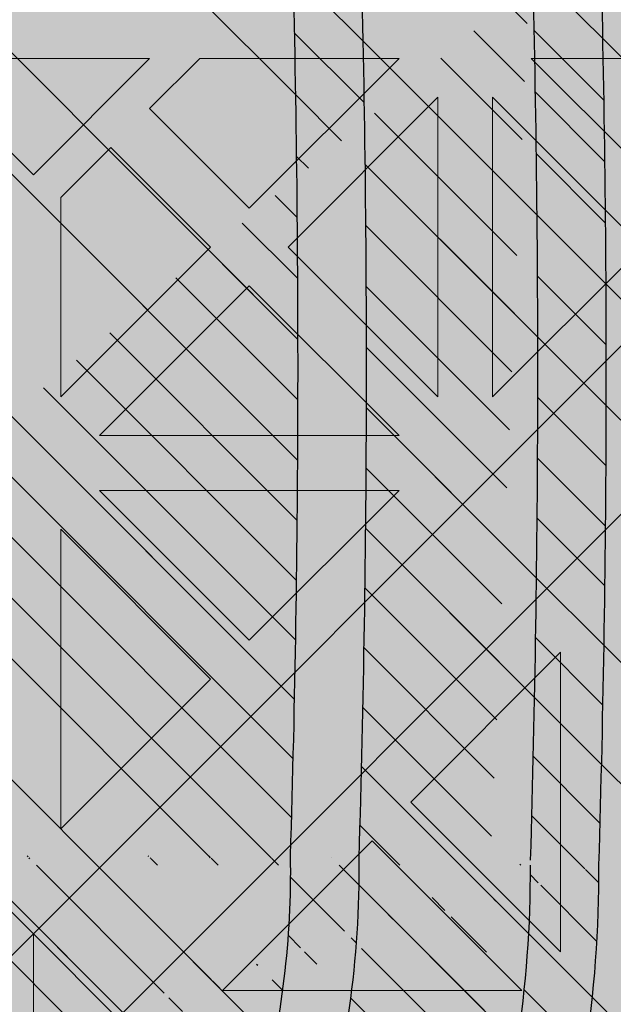
# Model space of a CAD drawing. Units: inches. Extents: x 844 to 2234, y 346 to 1084.
# Tile 28 of 93: x 1257.311 to 1260.074, y 691.183 to 695.763. Entities that reach past the tile are written whole.
import ezdxf

# ---------------------------------------------------------------- set-up
doc = ezdxf.new("R2010")
doc.units = ezdxf.units.IN
doc.header["$MEASUREMENT"] = 0
doc.layers.add('furniture', color=8, linetype='Continuous', lineweight=18)
doc.layers.add('RA-AP-01$0$INT', color=35, linetype='Continuous', lineweight=5)
doc.layers.add('RA-AP-01$0$FURN', color=3, linetype='Continuous')
doc.layers.add('RA-AP-01$0$WOOD', color=64, linetype='Continuous')

# ---------------------------------------------------------------- blocks, each defined once
blk = doc.blocks.new('A$C18D01794')
at = {"layer": 'RA-AP-01$0$INT'}
h = blk.add_hatch(color=256, dxfattribs=at)
h.paths.add_polyline_path([(4.585917135068449, -6.356712009588271), (4.555206456959269, -6.35671200958746), (4.555206456959137, -6.387422687716308), (4.874495778835233, -6.706712009592356), (4.90520645695423, -6.676001331474049)])
h.paths.add_polyline_path([(5.255206456948813, -6.387422687716306), (5.255206456948682, -6.356712009605972), (5.224495778822613, -6.356712009605161), (4.905206456953498, -6.676001331474273), (4.935917135072151, -6.706712009592924)])
h.paths.add_polyline_path([(4.935917135072559, -6.706712009592068), (4.905206456953564, -6.737422687710376), (5.255206456951813, -7.087422687708613), (5.255206456951549, -7.026001331471008)])
h.paths.add_polyline_path([(4.555206456956399, -7.026001331471013), (4.555206456956134, -7.087422687708616), (4.905206456953821, -6.737422687710943), (4.874495778835166, -6.70671200959229)])
h = blk.add_hatch(color=256, dxfattribs=at)
h.paths.add_polyline_path([(4.585917135068448, -6.356712009588273), (4.614201406330596, -6.356712009589021), (4.668846067270487, -6.411356670531338), (4.723490728212344, -6.356712009591912), (4.771774999457151, -6.35671200959319), (4.826419660396886, -6.411356670535356), (4.862780050090322, -6.374996280843536), (4.844495778842715, -6.356712009595112), (4.862780050090411, -6.356712009595595), (4.905206456960182, -6.399138416468211), (4.947632863832445, -6.356712009597838), (4.965917135079675, -6.356712009598322), (4.947632863831759, -6.374996280845421), (4.983993253523576, -6.411356670538857), (5.038637914464627, -6.356712009600247), (5.08692218571208, -6.356712009601523), (5.141566846649976, -6.411356670541852), (5.196211507589851, -6.356712009604411), (5.224495778822615, -6.356712009605161), (4.905206456953975, -6.676001331473793)])
h.paths.add_polyline_path([(4.895206456956031, -6.637717060225675), (4.895206456958921, -6.528427738347902), (4.840561796018589, -6.583072399285802)], flags=16)
h.paths.add_polyline_path([(4.915206456955638, -6.637717060226121), (4.969851117895509, -6.583072399288678), (4.915206456957609, -6.528427738348344)], flags=16)
h.paths.add_polyline_path([(4.826419660395175, -6.568930263661755), (4.881064321335613, -6.514285602723745), (4.771774999456703, -6.514285602720857)], flags=16)
h.paths.add_polyline_path([(4.983993253519558, -6.568930263665262), (5.038637914460456, -6.514285602726792), (4.929348592581548, -6.514285602724816)], flags=16)
h.paths.add_polyline_path([(4.881064321336025, -6.494285602723742), (4.826419660397532, -6.439640941782821), (4.771774999457062, -6.494285602720859)], flags=16)
h.paths.add_polyline_path([(4.929348592582019, -6.494285602724817), (5.038637914460982, -6.494285602726792), (4.983993253522945, -6.439640941786327)], flags=16)
h.paths.add_polyline_path([(4.895206456960191, -6.480143467100443), (4.895206456962115, -6.407422687715913), (4.876922185715016, -6.389138416467584), (4.840561796021581, -6.425498806159401)], flags=16)
h.paths.add_polyline_path([(4.915206456958487, -6.480143467100889), (4.969851117899527, -6.425498806162279), (4.933490728206909, -6.389138416468043), (4.9152064569598, -6.40742268771434)], flags=16)
h.paths.add_polyline_path([(4.757632863832376, -6.480143467096812), (4.812277524772842, -6.425498806158772), (4.757632863834348, -6.370854145217844)], flags=16)
h.paths.add_polyline_path([(4.737632863832376, -6.480143467096286), (4.737632863834348, -6.370854145217375), (4.682988202893906, -6.425498806155385)], flags=16)
h.paths.add_polyline_path([(5.05278005008503, -6.480143467103376), (5.052780050087917, -6.370854145224413), (4.998135389146995, -6.425498806162908)], flags=16)
h.paths.add_polyline_path([(5.072780050085024, -6.480143467103744), (5.127424711025931, -6.42549880616527), (5.072780050087916, -6.370854145224832)], flags=16)
h.paths.add_polyline_path([(4.935917135072783, -6.706712009592292), (5.255206456948811, -6.387422687716309), (5.255206456948932, -6.415706958964177), (5.200561796010279, -6.470351619902839), (5.255206456949403, -6.524996280841948), (5.25520645694961, -6.5732805520894), (5.200561796009787, -6.627925213029239), (5.236922185702417, -6.664285602721864), (5.255206456949919, -6.646001331474357), (5.255206456949998, -6.664285602721898), (5.212780050078687, -6.706712009592262), (5.25520645695036, -6.749138416463932), (5.255206456950438, -6.767422687711313), (5.236922185702424, -6.749138416463297), (5.200561796009796, -6.785498806155928), (5.255206456950753, -6.840143467096874), (5.25520645695096, -6.888427738341682), (5.200561796010322, -6.943072399282328), (5.255206456951428, -6.997717060223427), (5.255206456951547, -7.026001331471006)])
h.paths.add_polyline_path([(5.042988202883395, -6.785498806155427), (5.097632863823085, -6.840143467095101), (5.097632863822622, -6.730854145216193)], flags=16)
h.paths.add_polyline_path([(5.028846067259663, -6.771356670531693), (5.083490728198774, -6.716712009592573), (4.974201406321001, -6.716712009593042)], flags=16)
h.paths.add_polyline_path([(5.117632863823087, -6.840143467095186), (5.172277524762331, -6.785498806155926), (5.11763286382262, -6.730854145216225)], flags=16)
h.paths.add_polyline_path([(5.08349072819877, -6.696712009593886), (5.028846067259652, -6.642067348654775), (4.974201406320998, -6.696712009593438)], flags=16)
h.paths.add_polyline_path([(5.131774999446817, -6.854285602718917), (5.186419660386065, -6.799640941779662), (5.241064321325782, -6.854285602719365)], flags=17)
h.paths.add_polyline_path([(5.131774999446228, -6.716712009592374), (5.186419660386065, -6.771356670532194), (5.222780050079488, -6.734996280838764), (5.204495778832781, -6.716712009592063)], flags=16)
h.paths.add_polyline_path([(5.097632863822613, -6.682569873970264), (5.097632863823061, -6.573280552091354), (5.042988202883383, -6.627925213031044)], flags=16)
h.paths.add_polyline_path([(5.131774999446899, -6.874285602718915), (5.241064321325809, -6.874285602719364), (5.186419660386591, -6.928930263658598)], flags=17)
h.paths.add_polyline_path([(5.131774999446226, -6.696712009594078), (5.204495778830767, -6.696712009594374), (5.22278005007868, -6.67842773834687), (5.186419660386049, -6.642067348654249)], flags=16)
h.paths.add_polyline_path([(5.11763286382262, -6.682569873970225), (5.17227752476232, -6.627925213030515), (5.117632863823064, -6.573280552091267)], flags=16)
h.paths.add_polyline_path([(5.186419660386069, -6.613783077405491), (5.241064321325754, -6.559138416465795), (5.131774999446791, -6.559138416466263)], flags=16)
h.paths.add_polyline_path([(5.131774999446872, -6.539138416466263), (5.24106432132578, -6.539138416465794), (5.186419660386554, -6.484493755526573)], flags=16)
h.paths.add_polyline_path([(5.255206456951811, -7.08742268770861), (5.255206456951895, -7.106712009588038), (4.555206456956052, -7.106712009588038), (4.555206456956136, -7.087422687708617), (4.905206456953973, -6.737422687710788)])
h.paths.add_polyline_path([(4.983993253513404, -6.8444937555241), (4.92934859257295, -6.899138416462108), (5.03863791445186, -6.899138416465014)], flags=16)
h.paths.add_polyline_path([(4.969851117889988, -6.83035161990006), (4.915206456952556, -6.775706958960171), (4.915206456949648, -6.884996280837944)], flags=16)
h.paths.add_polyline_path([(4.929348592572535, -6.919138416462105), (4.983993253511019, -6.973783077403037), (5.038637914451496, -6.919138416465012)], flags=16)
h.paths.add_polyline_path([(5.052780050074912, -6.93328055208906), (4.998135389134438, -6.987925213027088), (5.052780050072919, -7.042569873968025)], flags=16)
h.paths.add_polyline_path([(5.07278005007491, -6.933280552089588), (5.072780050072918, -7.042569873968497), (5.127424711013374, -6.987925213030498)], flags=16)
h.paths.add_polyline_path([(4.89520645695295, -6.775706958959721), (4.840561796013067, -6.830351619897157), (4.895206456950961, -6.884996280837494)], flags=16)
h.paths.add_polyline_path([(4.915206456948365, -6.933280552085403), (4.915206456946434, -7.006001331471951), (4.933490728192729, -7.024285602719066), (4.969851117886972, -6.987925213026453)], flags=16)
h.paths.add_polyline_path([(4.881064321327021, -6.899138416461022), (4.82641966038902, -6.84449375552057), (4.771774999448108, -6.899138416459029)], flags=16)
h.paths.add_polyline_path([(4.895206456950073, -6.933280552084951), (4.840561796009022, -6.987925213023558), (4.876922185700835, -7.024285602716997), (4.895206456948749, -7.006001331469487)], flags=16)
h.paths.add_polyline_path([(4.983993253510392, -7.0020673486505), (4.947632863816944, -7.038427738342319), (4.965917135064043, -7.05671200959023), (5.038637914448995, -7.056712009591555)], flags=16)
h.paths.add_polyline_path([(4.881064321326543, -6.91913841646102), (4.771774999447578, -6.919138416459031), (4.826419660385607, -6.973783077399508)], flags=16)
h.paths.add_polyline_path([(4.905206456946447, -7.014285602717636), (4.862780050074785, -7.056712009588352), (4.947632863816685, -7.056712009589775)], flags=16)
h.paths.add_polyline_path([(5.14156684663679, -7.002067348654549), (5.086922185696452, -7.056712009592438), (5.196211507574223, -7.056712009594425)], flags=16)
h.paths.add_polyline_path([(4.8264196603837, -7.002067348646972), (4.771774999442643, -7.056712009585575), (4.8444957788276, -7.056712009587508), (4.862780050075511, -7.038427738340416)], flags=16)
h.paths.add_polyline_path([(4.812277524760289, -6.98792521302292), (4.757632863822258, -6.933280552082447), (4.757632863819352, -7.042569873961408)], flags=16)
h.paths.add_polyline_path([(4.73763286382226, -6.933280552082079), (4.682988202881349, -6.987925213020536), (4.737632863819352, -7.04256987396099)], flags=16)
h.paths.add_polyline_path([(4.723490728195188, -7.056712009584289), (4.668846067257299, -7.002067348643949), (4.614201406317417, -7.056712009581383)], flags=16)
h.paths.add_polyline_path([(4.597632863829262, -6.706712009592262), (4.555206456957951, -6.664285602721896), (4.555206456958029, -6.646001331474357), (4.573490728205535, -6.664285602721864), (4.609851117898167, -6.627925213029238), (4.555206456958338, -6.573280552089402), (4.555206456958546, -6.524996280841952), (4.60985111789767, -6.470351619902839), (4.555206456959015, -6.415706958964177), (4.555206456959138, -6.387422687716309), (4.874495778835167, -6.70671200959229), (4.5552064569564, -7.026001331471015), (4.555206456956523, -6.997717060223433), (4.609851117897629, -6.94307239928233), (4.555206456956988, -6.888427738341681), (4.555206456957198, -6.840143467096881), (4.609851117898153, -6.78549880615593), (4.573490728205528, -6.749138416463297), (4.555206456957507, -6.76742268771132), (4.555206456957585, -6.749138416463933)])
h.paths.add_polyline_path([(4.712780050085332, -6.730854145216195), (4.712780050084863, -6.840143467095105), (4.767424711024555, -6.785498806155427)], flags=16)
h.paths.add_polyline_path([(4.726922185709173, -6.716712009592573), (4.781566846648288, -6.771356670531693), (4.836211507586949, -6.716712009593043)], flags=16)
h.paths.add_polyline_path([(4.692780050085327, -6.730854145216225), (4.638135389145619, -6.785498806155928), (4.692780050084865, -6.840143467095185)], flags=16)
h.paths.add_polyline_path([(4.726922185709182, -6.696712009593886), (4.836211507586949, -6.696712009593436), (4.7815668466483, -6.642067348654773)], flags=16)
h.paths.add_polyline_path([(4.678637914461726, -6.71671200959237), (4.605917135075169, -6.716712009592063), (4.587632863828464, -6.734996280838766), (4.623993253521887, -6.771356670532195)], flags=16)
h.paths.add_polyline_path([(4.712780050085336, -6.68256987397026), (4.767424711024568, -6.627925213031042), (4.71278005008489, -6.573280552091352)], flags=16)
h.paths.add_polyline_path([(4.678637914461726, -6.696712009594076), (4.623993253521899, -6.642067348654247), (4.587632863829271, -6.67842773834687), (4.605917135077185, -6.696712009594376)], flags=16)
h.paths.add_polyline_path([(4.692780050085336, -6.682569873970228), (4.692780050084889, -6.573280552091267), (4.638135389145632, -6.627925213030515)], flags=16)
h.paths.add_polyline_path([(4.623993253521885, -6.799640941779662), (4.678637914461131, -6.854285602718915), (4.56934859258217, -6.854285602719365)], flags=17)
h.paths.add_polyline_path([(4.623993253521901, -6.613783077405509), (4.678637914461158, -6.559138416466263), (4.569348592582195, -6.559138416465795)], flags=16)
h.paths.add_polyline_path([(4.678637914461051, -6.874285602718915), (4.623993253521361, -6.928930263658598), (4.569348592582143, -6.874285602719364)], flags=17)
h.paths.add_polyline_path([(4.678637914461076, -6.539138416466263), (4.623993253521399, -6.484493755526573), (4.569348592582167, -6.539138416465796)], flags=16)
h = blk.add_hatch(color=256, dxfattribs=at)
h.paths.add_polyline_path([(4.781566846647504, -6.771356670530272), (4.836211507586161, -6.716712009591613), (4.726922185708388, -6.716712009591159)])
h.paths.add_polyline_path([(4.836211507586161, -6.696712009592008), (4.781566846647504, -6.642067348653354), (4.726922185708388, -6.69671200959247)])
h.paths.add_polyline_path([(4.76742471102377, -6.627925213029623), (4.712780050084083, -6.57328055208994), (4.712780050084542, -6.68256987396885)])
h.paths.add_polyline_path([(4.692780050084544, -6.682569873968819), (4.692780050084084, -6.573280552089856), (4.638135389144834, -6.627925213029111)])
h.paths.add_polyline_path([(4.678637914460932, -6.696712009592669), (4.623993253521102, -6.642067348652844), (4.587632863827676, -6.678427738346266), (4.605917135074382, -6.696712009592973)])
h.paths.add_polyline_path([(4.573490728204743, -6.664285602721736), (4.60985111789737, -6.627925213029108), (4.555206456957541, -6.573280552089279), (4.555206456957237, -6.646001331474231)])
h.paths.add_polyline_path([(4.623993253521098, -6.613783077405377), (4.67863791446035, -6.559138416466126), (4.56934859258139, -6.559138416465669)])
h.paths.add_polyline_path([(4.678637914460275, -6.539138416466126), (4.623993253520583, -6.48449375552644), (4.56934859258136, -6.539138416465672)])
h.paths.add_polyline_path([(4.609851117896854, -6.470351619902707), (4.555206456958196, -6.415706958964051), (4.555206456957738, -6.524996280841822)])
h.paths.add_polyline_path([(4.597632863828475, -6.706712009592775), (4.555206456957283, -6.664285602721582), (4.555206456956805, -6.749138416463489)])
h.paths.add_polyline_path([(4.678637914460932, -6.716712009590963), (4.605917135076396, -6.71671200959066), (4.587632863828479, -6.734996280838164), (4.623993253521104, -6.771356670530792)])
h.paths.add_polyline_path([(4.692780050084091, -6.840143467093776), (4.692780050084548, -6.730854145214809), (4.638135389144834, -6.785498806154524)])
h.paths.add_polyline_path([(4.767424711023772, -6.785498806154004), (4.712780050084545, -6.730854145214786), (4.712780050084089, -6.840143467093692)])
h.paths.add_polyline_path([(4.67863791446036, -6.854285602718778), (4.623993253521105, -6.799640941779527), (4.569348592581399, -6.854285602719237)])
h.paths.add_polyline_path([(4.609851117897371, -6.785498806155798), (4.573490728204743, -6.74913841646317), (4.555206456957237, -6.767422687710675), (4.555206456957548, -6.840143467095629)])
h.paths.add_polyline_path([(4.623993253520596, -6.928930263658465), (4.67863791446028, -6.874285602718778), (4.569348592581367, -6.874285602719238)])
h.paths.add_polyline_path([(4.609851117896867, -6.943072399282199), (4.555206456957749, -6.888427738343082), (4.55520645695821, -6.997717060220857)])
h = blk.add_hatch(color=256, dxfattribs=at)
h.paths.add_polyline_path([(4.905206456953579, -6.70671200959253), (4.905206456953751, -6.676001331474523), (4.874495778835229, -6.706712009592358)])
h.paths.add_polyline_path([(4.935917135071924, -6.706712009592703), (4.905206456953583, -6.706712009592529), (4.90520645695341, -6.737422687710532)])
h = blk.add_hatch(color=256, dxfattribs=at)
h.paths.add_polyline_path([(4.905206456953409, -6.737422687710532), (4.90520645695358, -6.706712009592529), (4.874495778835235, -6.706712009592359)])
h.paths.add_polyline_path([(4.935917135071928, -6.706712009592703), (4.905206456953754, -6.676001331474527), (4.905206456953582, -6.706712009592529)])
h = blk.add_hatch(color=256, dxfattribs=at)
h.paths.add_polyline_path([(4.895206456952951, -6.77570695895972), (4.840561796013068, -6.830351619897156), (4.895206456950958, -6.884996280837495)])
h.paths.add_polyline_path([(4.915206456949649, -6.884996280837942), (4.969851117889987, -6.830351619900054), (4.915206456952556, -6.775706958960171)])
h.paths.add_polyline_path([(5.038637914451862, -6.899138416465013), (4.983993253513403, -6.8444937555241), (4.929348592572953, -6.899138416462106)])
h.paths.add_polyline_path([(4.929348592572535, -6.919138416462105), (4.983993253511018, -6.973783077403037), (5.038637914451497, -6.919138416465012)])
h.paths.add_polyline_path([(4.915206456948366, -6.933280552085397), (4.915206456946433, -7.006001331471951), (4.93349072819273, -7.024285602719068), (4.969851117886972, -6.987925213026454)])
h.paths.add_polyline_path([(5.038637914448995, -7.056712009591553), (4.983993253510389, -7.002067348650502), (4.947632863816946, -7.038427738342318), (4.965917135064043, -7.05671200959023)])
h.paths.add_polyline_path([(5.05278005007292, -7.042569873968023), (5.05278005007491, -6.933280552089059), (4.998135389134438, -6.987925213027088)])
h.paths.add_polyline_path([(5.07278005007292, -7.042569873968496), (5.127424711013374, -6.987925213030498), (5.072780050074909, -6.933280552089588)])
h.paths.add_polyline_path([(5.141566846636789, -7.002067348654547), (5.086922185696449, -7.056712009592438), (5.196211507574223, -7.056712009594425)])
h.paths.add_polyline_path([(4.947632863816688, -7.056712009589774), (4.905206456946449, -7.014285602717634), (4.862780050074784, -7.056712009588353)])
h.paths.add_polyline_path([(4.840561796009025, -6.987925213023556), (4.876922185700834, -7.024285602716997), (4.895206456948747, -7.006001331469488), (4.895206456950075, -6.933280552084953)])
h.paths.add_polyline_path([(4.88106432132654, -6.919138416461021), (4.771774999447577, -6.919138416459031), (4.826419660385606, -6.973783077399508)])
h.paths.add_polyline_path([(4.881064321327019, -6.899138416461022), (4.826419660389019, -6.844493755520571), (4.771774999448108, -6.89913841645903)])
h.paths.add_polyline_path([(4.757632863819352, -7.042569873961409), (4.812277524760284, -6.987925213022922), (4.757632863822259, -6.933280552082447)])
h.paths.add_polyline_path([(4.8264196603837, -7.002067348646974), (4.771774999442646, -7.056712009585575), (4.844495778827599, -7.05671200958751), (4.862780050075512, -7.038427738340417)])
h.paths.add_polyline_path([(4.737632863819352, -7.042569873960988), (4.737632863822258, -6.933280552082078), (4.682988202881349, -6.987925213020538)])
h.paths.add_polyline_path([(4.668846067257299, -7.002067348643952), (4.61420140631742, -7.056712009581384), (4.723490728195189, -7.056712009584292)])
for p, q in [((4.905206456953753, -6.676001331474525), (4.905206456953409, -6.737422687710532)), ((4.874495778835167, -6.70671200959229), (4.555206456956399, -7.026001331471013)), ((4.874495778835233, -6.706712009592356), (4.905206456953409, -6.737422687710532)), ((4.935917135071927, -6.706712009592701), (4.905206456953407, -6.737422687710532)), ((4.726922185709178, -6.716712009592574), (4.836211507586949, -6.716712009593042)), ((4.72692218570918, -6.716712009592578), (4.781566846648288, -6.771356670531693)), ((4.836211507586949, -6.716712009593042), (4.781566846648288, -6.771356670531693)), ((4.712780050084865, -6.840143467095105), (4.71278005008533, -6.730854145216195)), ((4.71278005008533, -6.730854145216195), (4.767424711024555, -6.785498806155425)), ((4.905206456953975, -6.737422687710788), (4.555206456956136, -7.087422687708617)), ((4.905206456953975, -6.737422687710788), (5.255206456951811, -7.087422687708611)), ((4.89520645695295, -6.775706958959723), (4.840561796013068, -6.830351619897156)), ((4.895206456950959, -6.884996280837494), (4.89520645695295, -6.775706958959723)), ((4.767424711024554, -6.785498806155427), (4.712780050084865, -6.840143467095105)), ((4.895206456950956, -6.884996280837492), (4.840561796013068, -6.830351619897156)), ((4.826419660389018, -6.844493755520574), (4.771774999448109, -6.899138416459031)), ((4.881064321327019, -6.899138416461022), (4.82641966038902, -6.844493755520572)), ((4.771774999448109, -6.899138416459031), (4.881064321327019, -6.899138416461022)), ((4.771774999447578, -6.919138416459031), (4.881064321326541, -6.919138416461022)), ((4.771774999447578, -6.919138416459031), (4.826419660385606, -6.973783077399508)), ((4.881064321326541, -6.919138416461022), (4.826419660385606, -6.973783077399508)), ((4.682988202881351, -6.987925213020536), (4.737632863822258, -6.933280552082079)), ((4.737632863822258, -6.933280552082079), (4.737632863819352, -7.042569873960989)), ((4.757632863822258, -6.933280552082445), (4.812277524760285, -6.987925213022922)), ((4.757632863822258, -6.933280552082445), (4.757632863819352, -7.042569873961408)), ((4.895206456950073, -6.933280552084951), (4.840561796009024, -6.987925213023556)), ((4.895206456948748, -7.006001331469903), (4.895206456950073, -6.933280552084951)), ((4.737632863819352, -7.042569873960989), (4.682988202881349, -6.987925213020538)), ((4.757632863819352, -7.042569873961408), (4.812277524760285, -6.987925213022922)), ((4.840561796009024, -6.987925213023554), (4.876922185700835, -7.024285602716997)), ((4.723490728195186, -7.056712009584289), (4.668846067257299, -7.002067348643951)), ((4.771774999442645, -7.056712009585574), (4.8264196603837, -7.002067348646972)), ((4.826419660383698, -7.002067348646972), (4.862780050075511, -7.038427738340416)), ((4.895206456946431, -7.006001331471805), (4.876922185700835, -7.024285602716997)), ((4.905206456946449, -7.014285602717635), (4.862780050074783, -7.056712009588354)), ((4.905206456946449, -7.014285602717635), (4.94763286381669, -7.056712009589775)), ((4.844495778827597, -7.056712009587512), (4.862780050075513, -7.038427738340416)), ((4.723490728195188, -7.056712009584293), (4.614201406317417, -7.056712009581383)), ((4.844495778827597, -7.05671200958751), (4.771774999442645, -7.056712009585574)), ((4.94763286381669, -7.056712009589775), (4.862780050074783, -7.056712009588354))]:
    blk.add_line(p, q, dxfattribs=at)
blk = doc.blocks.new('A$C32926AE1')
at = {"layer": 'RA-AP-01$0$FURN'}
h = blk.add_hatch(dxfattribs=at)
h.set_pattern_fill('ANSI31', color=256, scale=0.1, style=0)
h.set_pattern_definition([(45, (0, 0), (-0.0088388347648318, 0.0088388347648318), [])])
edge = h.paths.add_edge_path(flags=16)
edge.add_arc((4.904771284329206, 4.246793130718756), 0.2603971832811541, 75.22398030683196, 104.7760196931204)
edge.add_arc((4.904771284329206, 4.246793130718756), 0.2603971832811541, 75.223980306832, 104.77601969312039, ccw=False)
edge = h.paths.add_edge_path(flags=16)
edge.add_arc((4.904771284329206, 4.067062675376612), 0.2603971832811541, 255.2239803068796, 284.776019693168)
edge.add_arc((4.904771284329206, 4.067062675376612), 0.2603971832811541, 255.22398030687958, 284.77601969316805, ccw=False)
edge = h.paths.add_edge_path(flags=0)
edge.add_arc((4.904771284329206, 4.067062675376612), 0.2603971832811541, 255.2239803068796, 284.776019693168)
edge.add_arc((4.904771284329206, 4.067062675376612), 0.2603971832811541, 255.22398030687958, 284.77601969316805, ccw=False)
edge = h.paths.add_edge_path(flags=0)
edge.add_arc((4.904771284329206, 4.067062675376612), 0.2603971832811541, 255.2239803068796, 284.776019693168)
edge.add_arc((4.904771284329206, 4.067062675376612), 0.2603971832811541, 255.22398030687958, 284.77601969316805, ccw=False)
edge = h.paths.add_edge_path()
edge.add_arc((4.604388392048174, 4.588829985554312), 0.1599999999999918, 342.3781640246255, 354.4317409793762)
edge.add_arc((5.090145208887507, 4.43216705527679), 0.3503971832811637, 162.0091218307731, 180.3186872093483)
edge.add_arc((5.205154176610243, 4.588829985554953), 0.1599999999999917, 185.5682590208461, 197.6218359767349)
edge.add_arc((4.904771284329229, 4.246793130718735), 0.3503971832811761, 72.00912183053516, 107.9908781690354)
edge.add_arc((9.535952835716557, 4.28682295566602), 4.798342501046485, 178.2875002453811, 181.5576802719453)
edge.add_arc((4.719397359771122, 4.43216705527679), 0.3503971832811637, 359.6813127906516, 377.9908781692269)
edge.add_arc((9.535967292294904, 4.286822350292874), 4.778371420254705, 178.2965938931842, 181.5667745797229)
edge.add_arc((4.719397359771122, 4.43216705527679), 0.3303971832811637, 359.6813127906516, 377.9908781692269)
edge.add_arc((0.2735752763637294, 4.286822350292874), 4.7783714202547, 358.4332254202771, 361.7034061068158)
edge.add_arc((5.061434214606998, 4.732549947558029), 0.1600000000000254, 252.3781640250584, 264.4317409792362)
edge.add_arc((4.748108354051257, 4.732549947558012), 0.1600000000000541, 275.5682590208426, 287.6218359759532)
edge.add_arc((4.604388392048115, 4.588829985554317), 0.1800000000000505, 342.3567572500182, 349.3735009646207)
edge.add_arc((5.205154176610254, 4.588829985554976), 0.1800000000000069, 190.6264990356027, 197.6432427513933)
edge.add_arc((5.061434214607106, 4.732549947558013), 0.1800000000000424, 252.3567572496606, 259.3735009644582)
edge.add_arc((4.904771284329208, 4.246793130718737), 0.3303971832811676, 71.99844483668534, 108.0015551637021)
edge.add_arc((4.748108354051414, 4.732549947558045), 0.1800000000000547, 280.6264990355479, 287.6432427495938)
edge.add_arc((5.090145208887514, 4.432167055276789), 0.2803971832811691, 162.8706300666893, 180.816523289902)
edge.add_arc((4.719397359771136, 4.432167055276689), 0.2803971832811534, 359.183476710103, 377.1293699333214)
edge.add_arc((4.904771284329222, 4.246793130718737), 0.2803971832811769, 72.87063006672916, 107.1293699332334)
edge.add_arc((5.090145208887522, 4.432167055276788), 0.2603971832811776, 165.2239803068007, 180.9953123810312)
edge.add_arc((4.719397359771141, 4.432167055276699), 0.2603971832811458, 359.0046876189768, 374.7760196932087)
edge.add_arc((5.090145208887507, 4.43216705527679), 0.3303971832811637, 162.0091218307731, 180.3186872093483)
edge.add_arc((9.53595427642584, 4.285015535491528), 4.728345371032053, 178.265043920078, 181.5679956281801)
edge.add_arc((0.2735882922327999, 4.285015535491582), 4.728345371032045, 358.4320043718193, 361.7349560799204)
edge.add_arc((9.535953591267507, 4.284458026472751), 4.708343996644348, 178.2573054306777, 181.5704995759608)
edge.add_arc((0.273588977391114, 4.284458026472785), 4.708343996644358, 358.4295004240388, 361.7426945693213)
edge.add_arc((0.2735889773911131, 4.029397779622582), 4.708343996644359, 358.2573054306787, 361.5704995759613)
edge.add_arc((9.535953591267518, 4.029397779622618), 4.708343996644359, 178.4295004240391, 181.7426945693223)
edge.add_arc((0.2735882922327901, 4.028840270603786), 4.728345371032054, 358.2650439200796, 361.5679956281808)
edge.add_arc((9.53595427642584, 4.028840270603841), 4.728345371032054, 178.4320043718199, 181.7349560799219)
edge.add_arc((0.2735752763637302, 4.027033455802493), 4.778371420254699, 358.2965938931842, 361.5667745797229)
edge.add_arc((4.719397359771122, 3.881688750818578), 0.3303971832811637, 342.0091218307731, 360.3186872093484)
edge.add_arc((5.090145208887507, 3.881688750818578), 0.3303971832811637, 179.6813127906516, 197.9908781692269)
edge.add_arc((9.535967292294904, 4.027033455802493), 4.778371420254705, 178.433225420277, 181.7034061068158)
edge.add_arc((4.719397359771122, 3.881688750818578), 0.3503971832811637, 342.0091218307731, 360.3186872093484)
edge.add_arc((9.53595283571655, 4.027032850429349), 4.79834250104648, 178.4423197280546, 181.7124997546188)
edge.add_arc((4.719397359771141, 3.881688750818669), 0.2603971832811458, 345.2239803067913, 360.9953123810232)
edge.add_arc((5.090145208887522, 3.88168875081858), 0.2603971832811776, 179.0046876189687, 194.7760196931993)
edge.add_arc((4.904771284329222, 4.067062675376631), 0.2803971832811769, 252.8706300667665, 287.1293699332708)
edge.add_arc((4.719397359771136, 3.881688750818678), 0.2803971832811534, 342.8706300666787, 360.8165232898969)
edge.add_arc((5.090145208887514, 3.881688750818579), 0.2803971832811691, 179.183476710098, 197.1293699333106)
edge.add_arc((4.748108354051414, 3.581305858537323), 0.1800000000000547, 72.3567572504062, 79.37350096445199)
edge.add_arc((4.904771284329208, 4.067062675376631), 0.3303971832811676, 251.9984448362979, 288.0015551633146)
edge.add_arc((5.061434214607106, 3.581305858537355), 0.1800000000000424, 100.6264990355418, 107.6432427503394)
edge.add_arc((5.205154176610254, 3.725025820540392), 0.1800000000000069, 162.3567572486066, 169.3735009643972)
edge.add_arc((4.604388392048115, 3.725025820541051), 0.1800000000000505, 10.62649903537925, 17.64324274998182)
edge.add_arc((4.748108354051257, 3.581305858537356), 0.1600000000000541, 72.37816402404681, 84.43174097915735)
edge.add_arc((4.904771284329229, 4.067062675376632), 0.3503971832811761, 252.0091218309645, 287.9908781694648)
edge.add_arc((5.061434214606998, 3.581305858537339), 0.1600000000000254, 95.56825902076373, 107.6218359749416)
edge.add_arc((5.205154176610243, 3.725025820540414), 0.1599999999999917, 162.3781640232651, 174.4317409791539)
edge.add_arc((5.090145208887507, 3.881688750818578), 0.3503971832811637, 179.6813127906516, 197.9908781692269)
edge.add_arc((4.604388392048174, 3.725025820541056), 0.1599999999999918, 5.568259020623824, 17.62183597537444)
edge.add_arc((0.2735897329420762, 4.28682295566602), 4.798342501046482, 358.4423197280547, 361.7124997546188)
edge.add_arc((0.2735897329420691, 4.027032850429348), 4.798342501046489, 358.2875002453812, 361.5576802719453)
at = {"layer": 'RA-AP-01$0$WOOD'}
h = blk.add_hatch(color=256, dxfattribs=at)
h.dxf.hatch_style = 1
h.paths.add_polyline_path([(5.157430609644524, 4.573483066760929, -0.1009492694046607), (5.155401577623758, 4.593365984175333, -0.1842662638101597), (5.172249623284174, 4.638795604568598, 0.2056608120311276), (5.179560981299304, 4.661316324430096, 0.3614336704623542), (5.134352340494423, 4.706524965234944, 0.2056608120311297), (5.111831620632933, 4.699213607219793, -0.1842662638101113), (5.066402000239693, 4.682365561559342, -0.1055311479399994), (5.045656153913092, 4.68467289944697, 0.1567636581983829), (4.763886414745334, 4.684672899446966, -0.1055311479399895), (4.743140568418733, 4.68236556155934, -0.1842662638100833), (4.6977109480255, 4.69921360721979, 0.2056608120302612), (4.675190228164109, 4.706524965234949, 0.3614336704708441), (4.629981587358889, 4.66131632442871, 0.2056608120245944), (4.637292945374126, 4.638795604567974, -0.1842662638101024), (4.654140991034615, 4.59336598417475, -0.1009492694055169), (4.652111959013835, 4.573483066760181, 0.021410119221476), (4.629748025606143, 4.156712009541676, 0.0214101192214795), (4.652111959013809, 3.739940952323101, -0.1009492694059586), (4.654140991034615, 3.720058034908448, -0.1842662638100975), (4.637292945374126, 3.674628414515226, 0.2056608120245705), (4.629981587358889, 3.652107694654492, 0.3614336704708879), (4.675190228164113, 3.606899053848249, 0.2056608120302384), (4.697710948025501, 3.614210411863408, -0.1842662638100995), (4.743140568418738, 3.63105845752386, -0.1055311479402541), (4.763886414745388, 3.628751119636215, 0.1567636581983776), (5.045656153913137, 3.628751119636244, -0.1055311479397538), (5.066402000239692, 3.631058457523857, -0.1842662638101067), (5.111831620632931, 3.614210411863407, 0.2056608120310924), (5.134352340494417, 3.606899053848256, 0.3614336704624001), (5.179560981299307, 3.652107694653103, 0.2056608120311314), (5.172249623284175, 3.6746284145146, -0.1842662638101402), (5.155401577623758, 3.72005803490786, -0.1009492694051366), (5.15743060964455, 3.739940952322354, 0.0214101192215073), (5.179794543052287, 4.156712009541468, 0.0214101192215252)])
h.paths.add_polyline_path([(4.639748609479751, 4.156712009541513, 0.0213537860821624), (4.661970494867118, 3.741887061152232, -0.094075836301374), (4.664143710413708, 3.7196126951003, -0.1824818158568985), (4.644813765429836, 3.668037719127816, 0.2056608120245319), (4.639939526753007, 3.653023905887301, 0.3614336704710246), (4.676106439397173, 3.616856993242342, 0.2056608120302234), (4.691120252638095, 3.621731231919122, -0.1824818158602558), (4.742695228611606, 3.641061176902986, -0.1029891339458722), (4.766991894714349, 3.638256818950944, 0.156709409989566), (5.042550673941472, 3.638256818950105, -0.102989133958497), (5.066847340047078, 3.641061176902949, -0.1824818158594995), (5.118422316020358, 3.621731231919103, 0.2056608120311416), (5.133436129261316, 3.616856993242346, 0.3614336704621468), (5.169603041905217, 3.653023905886178, 0.2056608120310986), (5.164728803228477, 3.668037719127177, -0.1824818158565612), (5.145398858244737, 3.719612695099578, -0.0940758363009313), (5.147572073791232, 3.741887061151398, 0.0213537860822023), (5.169793959178681, 4.156712009541451, 0.0213537860822226), (5.147572073791203, 4.571536957931898, -0.0940758363005034), (5.145398858244737, 4.59381132398362, -0.1824818158565587), (5.164728803228476, 4.645386299956021, 0.2056608120311045), (5.169603041905216, 4.66040011319702, 0.3614336704621845), (5.133436129261313, 4.696567025840856, 0.2056608120310773), (5.118422316020359, 4.691692787164098, -0.182481815859508), (5.066847340047078, 4.67236284218025, -0.1029891339584606), (5.04255067394148, 4.675167200133092, 0.156709409989566), (4.766991894714357, 4.675167200132257, -0.1029891339458842), (4.742695228611611, 4.672362842180213, -0.1824818158602725), (4.691120252638095, 4.691692787164077, 0.2056608120302152), (4.676106439397174, 4.696567025840858, 0.3614336704710363), (4.639939526753005, 4.660400113195899, 0.2056608120245495), (4.644813765429837, 4.645386299955384, -0.1824818158568934), (4.664143710413708, 4.593811323982902, -0.0940758363009187), (4.661970494867149, 4.571536957931074, 0.021353786082177)], flags=16)
h.paths.add_polyline_path([(5.129794543052235, 4.432167055276933, -0.0141661062790638), (5.130152669293814, 4.156927903047693, -0.0141661062790647), (5.129794543052234, 3.881688750818433, -0.0785247771143638), (5.10979738006795, 3.755143611847103, 0.0945969212073497), (5.105408519571111, 3.717898134952927, 0.1043170707844957), (5.116074640131521, 3.670385395016088, 0.1043170707864965), (5.068561900193738, 3.681051515576561, 0.09459692119553), (5.031316423304057, 3.676662655080835, -0.1580239521427272), (4.778226145355827, 3.676662655080367, 0.0945969211986668), (4.740980668464973, 3.681051515576592, 0.1043170707882822), (4.693467928526415, 3.670385395015844, 0.1043170707867916), (4.704134049087309, 3.717898134953662, 0.0945969211972894), (4.69974518859162, 3.755143611844042, -0.0785247771163196), (4.679748025606343, 3.881688750818406, -0.0141661062790663), (4.679389899364763, 4.156927903047693, -0.0141661062790672), (4.679748025606343, 4.432167055276998, -0.0785247771163064), (4.699745188591625, 4.55871219425134, 0.094596921197333), (4.704134049087308, 4.595957671141738, 0.1043170707867205), (4.693467928526416, 4.643470411079523, 0.1043170707882628), (4.740980668464965, 4.632804290518776, 0.0945969211988114), (4.778226145355874, 4.637193151015016, -0.158023952142669), (5.031316423304015, 4.637193151014546, 0.0945969211956361), (5.068561900193736, 4.632804290518806, 0.1043170707864979), (5.11607464013152, 4.643470411079278, 0.1043170707844617), (5.105408519571112, 4.595957671142455, 0.0945969212074597), (5.109797380067959, 4.558712194248236, -0.0785247771143467)], flags=0)
h.paths.add_polyline_path([(5.119794532311105, 4.432259799204851, -0.0142000800617244), (5.120156169157484, 4.156927903047701, -0.0142000800617277), (5.119794532311105, 3.881596006890482, -0.0784894509520253), (5.100273383573699, 3.758192358677797, 0.0940138827242913), (5.095413455884425, 3.717477693979438, 0.0606271852308753), (5.099615656341024, 3.686844378806616, 0.0606271852322524), (5.068982341167493, 3.691046579263239, 0.0940138827010453), (5.028267676478798, 3.686186651576848, -0.1580706864508061), (4.781274892180912, 3.686186651576435, 0.0940138827026903), (4.740560227491556, 3.691046579263279, 0.0606271852339895), (4.709926912317155, 3.686844378806508, 0.0606271852329405), (4.714129112773991, 3.717477693980356, 0.094013882701304), (4.709269185087677, 3.758192358669163, -0.0784894509577193), (4.689748036347473, 3.881596006890469, -0.014200080061729), (4.689386399501094, 4.156927903047709, -0.0142000800617217), (4.689748036347473, 4.432259799204808, -0.078489450957724), (4.709269185087651, 4.555663447426125, 0.0940138827014585), (4.714129112773992, 4.596378112114996, 0.0606271852329731), (4.709926912317154, 4.62701142728886, 0.0606271852340196), (4.74056022749157, 4.622809226832087, 0.0940138827024997), (4.781274892180847, 4.627669154518912, -0.1580706864508359), (5.028267676478777, 4.627669154518526, 0.0940138827010946), (5.068982341167492, 4.622809226832129, 0.060627185232254), (5.099615656341024, 4.627011427288751, 0.0606271852308727), (5.095413455884425, 4.59637811211593, 0.0940138827241088), (5.100273383573675, 4.555663447417647, -0.0784894509520978)], flags=0)
h.paths.add_polyline_path([(5.06978912287499, 4.430218106756144, -0.014241683694547), (5.070173729147532, 4.156927903047672, -0.0142416836945458), (5.06978912287499, 3.883637699339223, -0.0800609523125196), (5.052662118612511, 3.773463122773442, 0.0526421978001116), (5.04590916754064, 3.740550867606997, 0.0526421977992423), (5.012996912374707, 3.73379791653534, -0.1583028414718258), (4.796545656286308, 3.73379791653451, 0.0526421978034211), (4.763633401117837, 3.740550867607021, 0.0526421978018622), (4.756880450045755, 3.773463122774558, -0.0800609523117106), (4.739753445783639, 3.883637699339268, -0.0142416836945435), (4.739368839511098, 4.156927903047671, -0.0142416836945477), (4.739753445783639, 4.430218106756155, -0.0800609523116345), (4.75688045004574, 4.540392683320762, 0.052642197801941), (4.763633401117837, 4.573304938488346, 0.0526421978035071), (4.796545656286361, 4.580057889560873, -0.1583028414717561), (5.012996912374669, 4.580057889560039, 0.0526421977993048), (5.04590916754064, 4.57330493848837, 0.0526421978002057), (5.052662118612529, 4.540392683321868, -0.080060952312477)], flags=0)
h.paths.add_polyline_path([(5.049789715110557, 4.43038092723357, -0.0143097550741839), (5.05018085590259, 4.156927903047715, -0.0143097550741854), (5.049789715110558, 3.883474878861827, -0.0800685599149176), (5.03362098255317, 3.779581877367999, 0.0306258898956367), (5.028241146483733, 3.758218888663947, 0.0306258898977031), (5.006878157778253, 3.75283905259408, -0.1583983521624096), (4.802664410878162, 3.752839052594731, 0.0306258898946014), (4.781301422174808, 3.758218888663924, 0.0306258898967912), (4.775921586105202, 3.779581877368794, -0.080068559914251), (4.759752853548071, 3.883474878861786, -0.0143097550741854), (4.759361712756037, 4.156927903047671, -0.0143097550741854), (4.759752853548071, 4.430380927233557, -0.0800685599142479), (4.775921586105193, 4.534273928726546, 0.0306258898968306), (4.781301422174808, 4.555636917431444, 0.0306258898945754), (4.802664410878143, 4.561016753500631, -0.1583983521624168), (5.006878157778244, 4.561016753501291, 0.0306258898977177), (5.028241146483733, 4.555636917431421, 0.0306258898958182), (5.03362098255321, 4.534273928727244, -0.080068559914796)], flags=0)
h.paths.add_polyline_path([(4.999766070382627, 4.428171244713864, -0.0143443147609634), (5.000198441819402, 4.156927903047689, -0.0143443147609612), (4.999766070382627, 3.885684561381556, -0.0784641635803329), (4.987356730658798, 3.799103304488872, -0.1506053783831347), (4.822185837999821, 3.79910330448882, -0.0784641635803318), (4.809776498276007, 3.885684561381509, -0.014344314760963), (4.809344126839227, 4.156927903047677, -0.0143443147609645), (4.809776498276007, 4.428171244713873, -0.0784641635803192), (4.822185837999822, 4.514752501606549, -0.1506053783831338), (4.987356730658798, 4.514752501606494, -0.078464163580285)], flags=0)
h.paths.add_polyline_path([(4.979755254238824, 4.42764379880488, -0.0143772539198268), (4.980205517789977, 4.156927903047693, -0.0143772539198275), (4.979755254238824, 3.886212007290489, -0.0689242507424422), (4.971183264704897, 3.815276770442801, -0.1296645318904179), (4.838359303953726, 3.815276770442746, -0.0689242507424186), (4.829787314419809, 3.886212007290419, -0.0143772539198292), (4.829337050868653, 4.156927903047653, -0.0143772539198325), (4.829787314419809, 4.427643798804946, -0.0689242507424211), (4.838359303953725, 4.498579035652621, -0.1296645318904187), (4.971183264704897, 4.498579035652565, -0.0689242507424401)], flags=0)
h = blk.add_hatch(color=256, dxfattribs=at)
h.dxf.hatch_style = 1
h.paths.add_polyline_path([(5.145398858244737, 4.59381132398362, -0.1824818158565616), (5.164728803228476, 4.645386299956021, 0.2056608120311045), (5.169603041905216, 4.66040011319702, 0.3614336704621845), (5.133436129261313, 4.696567025840856, 0.2056608120310773), (5.118422316020359, 4.691692787164098, -0.182481815859508), (5.066847340047078, 4.67236284218025, -0.1029891339584606), (5.04255067394148, 4.675167200133092, 0.156709409989566), (4.766991894714357, 4.675167200132257, -0.1029891339458842), (4.742695228611611, 4.672362842180213, -0.1824818158602725), (4.691120252638095, 4.691692787164077, 0.2056608120302152), (4.676106439397174, 4.696567025840858, 0.3614336704710363), (4.639939526753005, 4.660400113195899, 0.2056608120245495), (4.644813765429837, 4.645386299955384, -0.1824818158568934), (4.664143710413708, 4.593811323982902, -0.0940758363009187), (4.661970494867149, 4.571536957931074, 0.0213537860821772), (4.639748609479751, 4.156712009541507, 0.0213537860821625), (4.661970494867119, 3.741887061152226, -0.0940758363013071), (4.664143710413708, 3.719612695100309, -0.1824818158569294), (4.644813765429836, 3.668037719127816, 0.2056608120245319), (4.639939526753007, 3.653023905887301, 0.3614336704710246), (4.676106439397173, 3.616856993242342, 0.2056608120302234), (4.691120252638095, 3.621731231919122, -0.1824818158602558), (4.742695228611606, 3.641061176902986, -0.1029891339458722), (4.766991894714349, 3.638256818950944, 0.156709409989566), (5.042550673941472, 3.638256818950105, -0.102989133958497), (5.066847340047078, 3.641061176902949, -0.1824818158594995), (5.118422316020358, 3.621731231919103, 0.2056608120311416), (5.133436129261316, 3.616856993242346, 0.3614336704621468), (5.169603041905217, 3.653023905886178, 0.2056608120310986), (5.164728803228477, 3.668037719127177, -0.1824818158565612), (5.145398858244737, 3.719612695099578, -0.0940758363009313), (5.147572073791232, 3.741887061151398, 0.0213537860822023), (5.169793959178681, 4.156712009541451, 0.0213537860822226), (5.147572073791203, 4.571536957931898, -0.0940758363004996)])
h.paths.add_polyline_path([(5.109797380067958, 4.55871219424824, -0.0785247771143472), (5.129794543052234, 4.432167055276936, -0.0141661062790644), (5.130152669293814, 4.156927903047685, -0.014166106279066), (5.129794543052234, 3.881688750818401, -0.0785247771143517), (5.109797380067946, 3.755143611847092, 0.0945969212073132), (5.105408519571111, 3.717898134952929, 0.1043170707844995), (5.116074640131521, 3.670385395016088, 0.1043170707864965), (5.068561900193738, 3.681051515576561, 0.09459692119553), (5.031316423304057, 3.676662655080835, -0.1580239521427272), (4.778226145355827, 3.676662655080367, 0.0945969211986668), (4.740980668464973, 3.681051515576592, 0.1043170707882822), (4.693467928526415, 3.670385395015844, 0.1043170707867916), (4.704134049087309, 3.717898134953662, 0.0945969211972894), (4.69974518859162, 3.755143611844042, -0.0785247771163196), (4.679748025606343, 3.881688750818406, -0.0141661062790663), (4.679389899364763, 4.156927903047693, -0.0141661062790672), (4.679748025606343, 4.432167055276998, -0.0785247771163064), (4.699745188591625, 4.55871219425134, 0.094596921197333), (4.704134049087308, 4.595957671141738, 0.1043170707867205), (4.693467928526416, 4.643470411079523, 0.1043170707882628), (4.740980668464965, 4.632804290518776, 0.0945969211988114), (4.778226145355874, 4.637193151015016, -0.158023952142669), (5.031316423304015, 4.637193151014546, 0.0945969211956361), (5.068561900193736, 4.632804290518806, 0.1043170707864979), (5.11607464013152, 4.643470411079278, 0.1043170707844617), (5.105408519571112, 4.595957671142455, 0.0945969212074504)], flags=16)
h.paths.add_polyline_path([(5.100273383573655, 4.55566344741771, -0.0784894509521388), (5.119794532311105, 4.432259799204852, -0.0142000800617252), (5.120156169157484, 4.156927903047686, -0.014200080061726), (5.119794532311105, 3.881596006890502, -0.0784894509520446), (5.100273383573696, 3.758192358677786, 0.0940138827242721), (5.095413455884425, 3.717477693979436, 0.0606271852308692), (5.099615656341024, 3.686844378806616, 0.0606271852322522), (5.068982341167493, 3.691046579263239, 0.0940138827010453), (5.028267676478798, 3.686186651576848, -0.1580706864508061), (4.781274892180912, 3.686186651576435, 0.0940138827026903), (4.740560227491556, 3.691046579263279, 0.0606271852339895), (4.709926912317155, 3.686844378806508, 0.0606271852329405), (4.714129112773991, 3.717477693980356, 0.094013882701304), (4.709269185087677, 3.758192358669163, -0.0784894509577193), (4.689748036347473, 3.881596006890469, -0.014200080061729), (4.689386399501094, 4.156927903047709, -0.0142000800617217), (4.689748036347473, 4.432259799204808, -0.078489450957724), (4.709269185087651, 4.555663447426125, 0.0940138827014585), (4.714129112773992, 4.596378112114996, 0.0606271852329731), (4.709926912317154, 4.62701142728886, 0.0606271852340196), (4.74056022749157, 4.622809226832087, 0.0940138827024997), (4.781274892180847, 4.627669154518912, -0.1580706864508359), (5.028267676478777, 4.627669154518526, 0.0940138827010946), (5.068982341167492, 4.622809226832129, 0.060627185232254), (5.099615656341024, 4.627011427288751, 0.0606271852308727), (5.095413455884425, 4.59637811211593, 0.094013882723957)], flags=0)
h.paths.add_polyline_path([(5.04590916754064, 4.57330493848837, 0.0526421978002057), (5.052662118612529, 4.540392683321868, -0.0800609523124783), (5.06978912287499, 4.430218106756142, -0.0142416836945469), (5.070173729147532, 4.156927903047672, -0.0142416836945458), (5.06978912287499, 3.883637699339223, -0.0800609523125196), (5.052662118612511, 3.773463122773442, 0.0526421978001116), (5.04590916754064, 3.740550867606997, 0.0526421977992423), (5.012996912374707, 3.73379791653534, -0.1583028414718258), (4.796545656286308, 3.73379791653451, 0.0526421978034211), (4.763633401117837, 3.740550867607021, 0.0526421978018622), (4.756880450045755, 3.773463122774558, -0.0800609523117106), (4.739753445783639, 3.883637699339268, -0.0142416836945435), (4.739368839511098, 4.156927903047671, -0.0142416836945477), (4.739753445783639, 4.430218106756155, -0.0800609523116345), (4.75688045004574, 4.540392683320762, 0.052642197801941), (4.763633401117837, 4.573304938488346, 0.0526421978035071), (4.796545656286361, 4.580057889560873, -0.1583028414717561), (5.012996912374669, 4.580057889560039, 0.0526421977993048)], flags=0)
h.paths.add_polyline_path([(5.028241146483733, 4.555636917431422, 0.0306258898956949), (5.033620982553182, 4.534273928727329, -0.0800685599148649), (5.049789715110557, 4.430380927233569, -0.0143097550741839), (5.05018085590259, 4.156927903047715, -0.0143097550741854), (5.049789715110558, 3.883474878861827, -0.0800685599149176), (5.03362098255317, 3.779581877367999, 0.0306258898956367), (5.028241146483733, 3.758218888663947, 0.0306258898977031), (5.006878157778253, 3.75283905259408, -0.1583983521624096), (4.802664410878162, 3.752839052594731, 0.0306258898946014), (4.781301422174808, 3.758218888663924, 0.0306258898967912), (4.775921586105202, 3.779581877368794, -0.080068559914251), (4.759752853548071, 3.883474878861786, -0.0143097550741854), (4.759361712756037, 4.156927903047671, -0.0143097550741854), (4.759752853548071, 4.430380927233557, -0.0800685599142479), (4.775921586105193, 4.534273928726546, 0.0306258898968306), (4.781301422174808, 4.555636917431444, 0.0306258898945754), (4.802664410878143, 4.561016753500631, -0.1583983521624168), (5.006878157778244, 4.561016753501291, 0.0306258898977174)], flags=0)
h.paths.add_polyline_path([(4.987356730658798, 4.514752501606494, -0.0784641635803018), (4.999766070382627, 4.428171244713845, -0.0143443147609637), (5.000198441819402, 4.156927903047665, -0.0143443147609622), (4.999766070382628, 3.885684561381514, -0.0784641635802952), (4.987356730658797, 3.799103304488872, -0.1506053783831338), (4.822185837999821, 3.799103304488819, -0.0784641635803342), (4.809776498276007, 3.885684561381512, -0.0143443147609628), (4.809344126839227, 4.156927903047676, -0.0143443147609646), (4.809776498276007, 4.428171244713873, -0.0784641635803192), (4.822185837999822, 4.514752501606549, -0.1506053783831338)], flags=0)
h.paths.add_polyline_path([(4.971183264704897, 4.498579035652566, -0.0689242507424384), (4.979755254238824, 4.427643798804883, -0.0143772539198276), (4.980205517789977, 4.15692790304768, -0.0143772539198258), (4.979755254238823, 3.88621200729051, -0.0689242507424628), (4.971183264704897, 3.815276770442801, -0.129664531890417), (4.838359303953726, 3.815276770442746, -0.0689242507424186), (4.829787314419809, 3.886212007290419, -0.0143772539198292), (4.829337050868653, 4.156927903047653, -0.0143772539198325), (4.829787314419809, 4.427643798804946, -0.0689242507424211), (4.838359303953725, 4.498579035652621, -0.1296645318904187)], flags=0)
h = blk.add_hatch(dxfattribs=at)
h.set_pattern_fill('ANSI31', color=256, scale=0.05, style=0)
h.set_pattern_definition([(45, (0, 0), (-0.0044194173824159, 0.0044194173824159), [])])
h.paths.add_polyline_path([(5.130152669293814, 4.156927903047704, 0.0141661062790657), (5.129794543052234, 4.432167055276982, 0.0777827904001433), (5.110168979996553, 4.557559993161921, -0.0976515123401879), (5.105408519571111, 4.595957671142454, -0.1043170707844687), (5.116074640131522, 4.64347041107928), (5.099615656341024, 4.627011427288751, 0.0606271852308727), (5.095413455884425, 4.59637811211593, 0.0940138827241088), (5.100273383573675, 4.555663447417647, -0.0784894509520972), (5.119794532311105, 4.432259799204852, -0.0142000800617252), (5.120156169157484, 4.156927903047686, -0.014200080061726), (5.119794532311105, 3.881596006890502, -0.0784894509520446), (5.100273383573696, 3.758192358677786, 0.0940138827242721), (5.095413455884425, 3.717477693979436, 0.0606271852308692), (5.099615656341024, 3.686844378806616), (5.116074640131519, 3.67038539501609, -0.1043170707844594), (5.105408519571112, 3.717898134952912, -0.0976515123401594), (5.11016897999655, 3.756295812933435, 0.0777827904001654), (5.129794543052234, 3.881688750818409, 0.0141661062790665)])
h.paths.add_polyline_path([(5.030164222210597, 3.676291055149937, -0.0976515123472002), (5.068561900193739, 3.681051515576561, -0.1043170707864927), (5.116074640131521, 3.670385395016088), (5.099615656341024, 3.686844378806616, 0.0606271852322522), (5.068982341167493, 3.691046579263239, 0.0940138827010453), (5.028267676478798, 3.686186651576848, -0.1580706864508061), (4.781274892180912, 3.686186651576435, 0.0940138827026903), (4.740560227491556, 3.691046579263279, 0.0606271852339913), (4.709926912317154, 3.686844378806508), (4.693467928526416, 3.670385395015845, -0.1043170707882796), (4.740980668464973, 3.681051515576592, -0.0976515123427246), (4.779378346446416, 3.676291055150394, 0.156512506893803)])
h.paths.add_polyline_path([(4.689748036347473, 3.881596006890472, -0.014200080061729), (4.689386399501094, 4.156927903047712, -0.0142000800617195), (4.689748036347473, 4.432259799204768, -0.078489450957742), (4.709269185087648, 4.555663447426114, 0.0940138827014821), (4.714129112773992, 4.596378112114995, 0.0606271852329748), (4.709926912317154, 4.62701142728886), (4.693467928526414, 4.643470411079524, -0.1043170707867939), (4.704134049087309, 4.595957671141706, -0.09765151234893), (4.699373588660725, 4.557559993157876, 0.0777827903975372), (4.679748025606343, 4.432167055276987, 0.0141661062790675), (4.679389899364763, 4.156927903047675, 0.0141661062790641), (4.679748025606343, 3.88168875081843, 0.0777827903975637), (4.699373588660724, 3.756295812937497, -0.0976515123490278), (4.704134049087308, 3.717898134953629, -0.1043170707867196), (4.693467928526416, 3.670385395015845), (4.709926912317155, 3.686844378806508, 0.0606271852329413), (4.714129112773991, 3.717477693980357, 0.0940138827013084), (4.709269185087676, 3.758192358669166, -0.0784894509577192)])
h.paths.add_polyline_path([(4.779378346446434, 4.63756475094498, -0.0976515123427943), (4.740980668464964, 4.632804290518776, -0.1043170707882609), (4.693467928526416, 4.643470411079523), (4.709926912317154, 4.62701142728886, 0.0606271852340196), (4.74056022749157, 4.622809226832087, 0.0940138827024997), (4.781274892180847, 4.627669154518912, -0.1580706864508359), (5.028267676478777, 4.627669154518526, 0.0940138827010946), (5.068982341167492, 4.622809226832129, 0.060627185232254), (5.099615656341024, 4.627011427288751), (5.116074640131521, 4.643470411079279, -0.1043170707865022), (5.068561900193735, 4.632804290518806, -0.0976515123475899), (5.030164222210446, 4.637564750945479, 0.1565125068936924)])
h = blk.add_hatch(dxfattribs=at)
h.set_pattern_fill('ANSI32', color=256, scale=0.2, style=0)
h.set_pattern_definition([(45, (0, 0), (-0.0530330085889911, 0.0530330085889911), []), (45, (0.035355339, 0), (-0.0530330085889911, 0.0530330085889911), [])])
h.paths.add_polyline_path([(5.119794532311105, 4.432259799204823, 0.0777015974868765), (5.10065834347252, 4.554469821747928, -0.0968902511992216), (5.095413455884425, 4.596378112115931, -0.060627185230871), (5.099615656341024, 4.627011427288751, -0.060627185232254), (5.068982341167492, 4.622809226832129, -0.0968902512198245), (5.027074050790956, 4.628054114423209, 0.1564657949319105), (4.782468517866163, 4.628054114422785, -0.0968902512152247), (4.740560227491555, 4.622809226832088, -0.0606271852339878), (4.709926912317155, 4.627011427288859, -0.0606271852329413), (4.714129112773991, 4.596378112115011, -0.0968902512205338), (4.708884225182929, 4.554469821738175, 0.0777015974804443), (4.689748036347473, 4.43225979920482, 0.0142000800617215), (4.689386399501094, 4.156927903047726, 0.0142000800617273), (4.689748036347473, 3.88159600689052, 0.077701597480541), (4.708884225182985, 3.759385984357019, -0.096890251220082), (4.714129112773992, 3.717477693980371, -0.0606271852329731), (4.709926912317154, 3.686844378806507, -0.060627185233988), (4.740560227491554, 3.691046579263279, -0.0968902512152569), (4.782468517866175, 3.685801691672578, 0.1564657949319236), (5.027074050790988, 3.685801691672169, -0.0968902512197451), (5.068982341167491, 3.691046579263239, -0.0606271852322557), (5.099615656341024, 3.686844378806616, -0.0606271852308727), (5.095413455884425, 3.717477693979438, -0.0968902511991229), (5.100658343472507, 3.7593859843474, 0.0777015974868745), (5.119794532311105, 3.8815960068905, 0.014200080061726), (5.120156169157484, 4.156927903047685, 0.0142000800617238)])
h.paths.add_polyline_path([(5.070173729147531, 4.156927903047684, -0.0142416836945481), (5.06978912287499, 3.883637699339191, -0.0800609523125107), (5.052662118612505, 3.773463122773424, 0.0526421978000811), (5.04590916754064, 3.740550867606997, 0.0526421977993214), (5.012996912374658, 3.733797916535325, -0.1583028414717916), (4.796545656286304, 3.733797916534512, 0.0526421978034138), (4.763633401117837, 3.740550867607021, 0.0526421978018622), (4.756880450045755, 3.773463122774558, -0.0800609523117106), (4.739753445783639, 3.883637699339268, -0.0142416836945435), (4.739368839511098, 4.156927903047671, -0.0142416836945477), (4.739753445783639, 4.430218106756155, -0.0800609523116345), (4.75688045004574, 4.540392683320762, 0.052642197801941), (4.763633401117837, 4.573304938488346, 0.0526421978035071), (4.796545656286361, 4.580057889560873, -0.1583028414717561), (5.012996912374669, 4.580057889560039, 0.0526421977993048), (5.04590916754064, 4.57330493848837, 0.0526421978002057), (5.052662118612529, 4.540392683321868, -0.0800609523124783), (5.06978912287499, 4.430218106756142, -0.0142416836945463)], flags=16)
h.paths.add_polyline_path([(5.050180855902591, 4.156927903047686, -0.0143097550741856), (5.049789715110558, 3.883474878861795, -0.0800685599148126), (5.033620982553202, 3.7795818773681, 0.0306258898957837), (5.028241146483733, 3.758218888663947, 0.0306258898977031), (5.006878157778253, 3.75283905259408, -0.1583983521624096), (4.802664410878162, 3.752839052594731, 0.0306258898946014), (4.781301422174808, 3.758218888663924, 0.0306258898967912), (4.775921586105202, 3.779581877368794, -0.080068559914251), (4.759752853548071, 3.883474878861786, -0.0143097550741854), (4.759361712756037, 4.156927903047671, -0.0143097550741854), (4.759752853548071, 4.430380927233557, -0.0800685599142479), (4.775921586105193, 4.534273928726546, 0.0306258898968306), (4.781301422174808, 4.555636917431444, 0.0306258898945754), (4.802664410878143, 4.561016753500631, -0.1583983521624168), (5.006878157778244, 4.561016753501291, 0.0306258898977177), (5.028241146483733, 4.555636917431421, 0.0306258898958182), (5.03362098255321, 4.534273928727244, -0.0800685599147973), (5.049789715110557, 4.430380927233568, -0.0143097550741854)], flags=0)
h.paths.add_polyline_path([(5.000198441819402, 4.15692790304769, -0.0143443147609622), (4.999766070382627, 3.885684561381539, -0.0784641635803169), (4.987356730658798, 3.799103304488873, -0.1506053783831347), (4.822185837999821, 3.79910330448882, -0.0784641635803318), (4.809776498276007, 3.885684561381509, -0.014344314760963), (4.809344126839227, 4.156927903047677, -0.0143443147609645), (4.809776498276007, 4.428171244713873, -0.0784641635803192), (4.822185837999822, 4.514752501606549, -0.1506053783831338), (4.987356730658798, 4.514752501606494, -0.0784641635803018), (4.999766070382627, 4.428171244713845, -0.0143443147609624)], flags=0)
h.paths.add_polyline_path([(4.980205517789976, 4.156927903047707, -0.0143772539198295), (4.979755254238824, 3.886212007290466, -0.06892425074242), (4.971183264704897, 3.815276770442801, -0.129664531890417), (4.838359303953726, 3.815276770442746, -0.0689242507424186), (4.829787314419809, 3.886212007290419, -0.0143772539198292), (4.829337050868653, 4.156927903047653, -0.0143772539198325), (4.829787314419809, 4.427643798804946, -0.0689242507424211), (4.838359303953725, 4.498579035652621, -0.1296645318904187), (4.971183264704897, 4.498579035652565, -0.0689242507424418), (4.979755254238824, 4.427643798804878, -0.0143772539198259)], flags=0)
for centre, radius, start, end in [((9.53595283571655, 4.027032850429349), 4.79834250104648, 178.4423197280546, 181.7124997546188), ((9.535967292294904, 4.027033455802493), 4.778371420254705, 178.433225420277, 181.7034061068158), ((9.53595427642584, 4.028840270603841), 4.728345371032054, 178.4320043718199, 181.7349560799219), ((9.535953591267518, 4.029397779622618), 4.708343996644359, 178.4295004240391, 181.7426945693223), ((5.090145208887514, 3.881688750818579), 0.2803971832811691, 179.183476710098, 197.1293699333106), ((5.090145208887522, 3.88168875081858), 0.2603971832811776, 179.0046876189687, 194.7760196931993), ((5.090145208887507, 3.881688750818578), 0.3503971832811637, 179.6813127906516, 197.9908781692269), ((5.090145208887507, 3.881688750818578), 0.3303971832811637, 179.6813127906516, 197.9908781692269)]:
    blk.add_arc(centre, radius, start, end, dxfattribs=at)
blk = doc.blocks.new('A$C5D2F253E')
at = {"layer": 'RA-AP-01$0$FURN', "xscale": -0.7999999999883585, "yscale": 0.7999999999883585, "zscale": 0.8, "rotation": 90}
blk.add_blockref('A$C18D01794', (-5.687757199772477, 4.75791982714071), dxfattribs=at)
at = {"layer": 'RA-AP-01$0$WOOD', "rotation": 270}
blk.add_blockref('A$C32926AE1', (-4.161339601644158, 5.73852594588169), dxfattribs=at)

msp = doc.modelspace()

# ---------------------------------------------------------------- block references
at = {"layer": 'furniture', "xscale": -15.94108302203742, "yscale": 15.94108302203742, "zscale": 15.94108302203742, "rotation": 270}
msp.add_blockref('A$C5D2F253E', (1244.08405109492, 696.2584716700112), dxfattribs=at)

doc.saveas('drawing.dxf')
